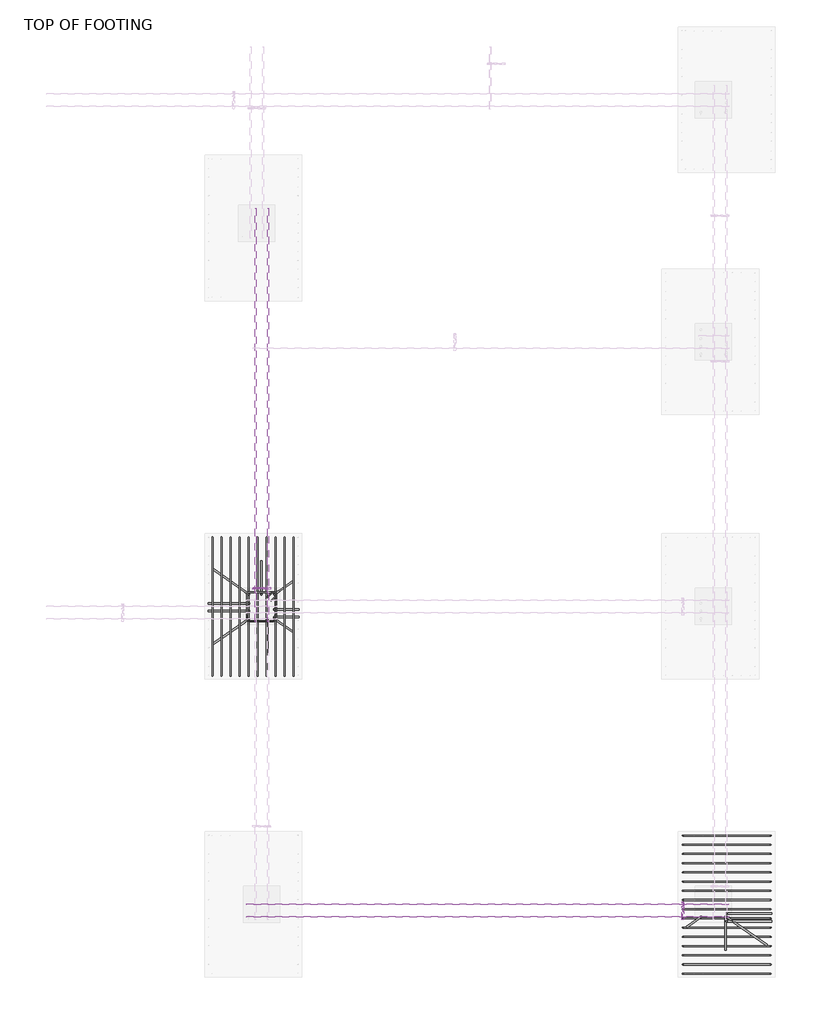
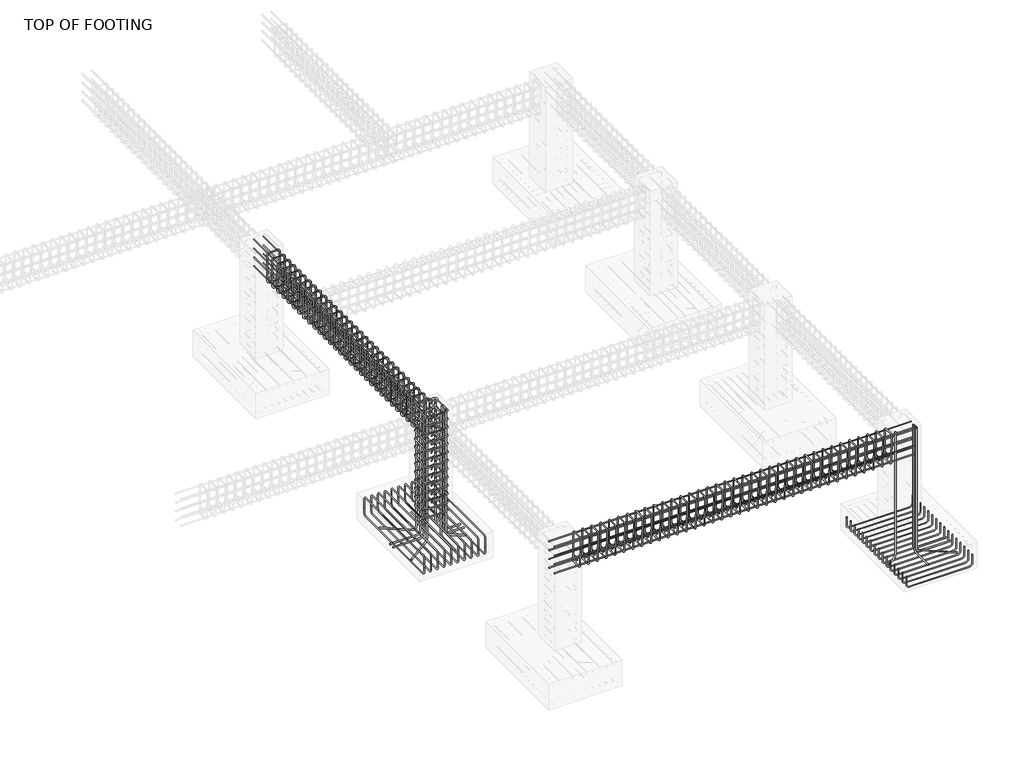
# One storey, part 4 of 11: 22 reinforcing bars.
"""IFC4 building model written with IfcOpenShell, lengths in millimetres."""

from ifc_helpers import new_model, si_unit, point, frame, origin, place, context, project, spatial, polyline, circle_curve, trimmed, segment, composite_curve, source, transform, mapped, element, save
from ifc_brep_helpers import swept_disk

model = new_model("IFC4")

# Units and contexts
model_context = context("Model", 3, world=origin())
ifc_project = project(units=[si_unit("LENGTHUNIT", "METRE", prefix="MILLI")], contexts=[model_context])

# Site, building, storey
site = spatial("IfcSite", under=ifc_project)
building = spatial("IfcBuilding", under=site)
storey = spatial("IfcBuildingStorey", under=building, Name="TOP OF FOOTING", Elevation=-1828.8)

# Reinforcing bars
placement = place(None, origin())
reinforcing_bar_shape = source(origin(), model_context, "Body", "SolidModel", [
    swept_disk(composite_curve([segment(polyline([(-1859.9394572, -2335.4013044, -2084.0984403), (-1859.9394572, -2335.4013044, -1936.7984403)]), True, "CONTINUOUS"), segment(trimmed(circle_curve(frame((-1859.9394572, -2381.7513044, -1936.7984403), z_axis=(1.0, 0.0, 0.0), x_axis=(0.0, 46.350000000000364, 0.0)), 46.35), [point((-1859.9394572, -2335.4013044, -1936.7984403))], [point((-1859.9394572, -2381.7513044, -1890.4484403))], True, "CARTESIAN"), True, "CONTINUOUS"), segment(polyline([(-1859.9394572, -2381.7513044, -1890.4484403), (-1859.9394572, -3996.3513044, -1890.4484403)]), True, "CONTINUOUS"), segment(trimmed(circle_curve(frame((-1859.9394572, -3996.3513044, -1936.7984403), z_axis=(1.0, 0.0, 0.0), x_axis=(0.0, 0.0, 46.350000000000136)), 46.35), [point((-1859.9394572, -3996.3513044, -1890.4484403))], [point((-1859.9394572, -4042.7013044, -1936.7984403))], True, "CARTESIAN"), True, "CONTINUOUS"), segment(polyline([(-1859.9394572, -4042.7013044, -1936.7984403), (-1859.9394572, -4042.7013044, -2084.0984403)]), True, "CONTINUOUS")], self_intersect=False), 6.35),
])
element("IfcReinforcingBar", 1, at=placement, inside=storey, context=model_context, shape_type="MappedRepresentation", body=[
    mapped(reinforcing_bar_shape, transform((0.0, 0.0, 0.0), x_axis=(1.0, 0.0, 0.0), y_axis=(0.0, 1.0, 0.0), z_axis=(0.0, 0.0, 1.0))),
    mapped(reinforcing_bar_shape, transform((-111.55177, 0.0, 0.0), x_axis=(1.0, 0.0, 0.0), y_axis=(0.0, 1.0, 0.0), z_axis=(0.0, 0.0, 1.0))),
    mapped(reinforcing_bar_shape, transform((-223.10354, 0.0, 0.0), x_axis=(1.0, 0.0, 0.0), y_axis=(0.0, 1.0, 0.0), z_axis=(0.0, 0.0, 1.0))),
    mapped(reinforcing_bar_shape, transform((-334.6553099, 0.0, 0.0), x_axis=(1.0, 0.0, 0.0), y_axis=(0.0, 1.0, 0.0), z_axis=(0.0, 0.0, 1.0))),
    mapped(reinforcing_bar_shape, transform((-446.2070799, 0.0, 0.0), x_axis=(1.0, 0.0, 0.0), y_axis=(0.0, 1.0, 0.0), z_axis=(0.0, 0.0, 1.0))),
    mapped(reinforcing_bar_shape, transform((-557.7588499, 0.0, 0.0), x_axis=(1.0, 0.0, 0.0), y_axis=(0.0, 1.0, 0.0), z_axis=(0.0, 0.0, 1.0))),
    mapped(reinforcing_bar_shape, transform((-669.3106199, 0.0, 0.0), x_axis=(1.0, 0.0, 0.0), y_axis=(0.0, 1.0, 0.0), z_axis=(0.0, 0.0, 1.0))),
    mapped(reinforcing_bar_shape, transform((-780.8623899, 0.0, 0.0), x_axis=(1.0, 0.0, 0.0), y_axis=(0.0, 1.0, 0.0), z_axis=(0.0, 0.0, 1.0))),
    mapped(reinforcing_bar_shape, transform((-892.4141599, 0.0, 0.0), x_axis=(1.0, 0.0, 0.0), y_axis=(0.0, 1.0, 0.0), z_axis=(0.0, 0.0, 1.0))),
    mapped(reinforcing_bar_shape, transform((-1003.9659298, 0.0, 0.0), x_axis=(1.0, 0.0, 0.0), y_axis=(0.0, 1.0, 0.0), z_axis=(0.0, 0.0, 1.0))),
])
reinforcing_bar_2_shape = source(origin(), model_context, "Body", "SolidModel", [
    swept_disk(composite_curve([segment(polyline([(-2863.9053871, -2335.4013044, -2021.5298587), (-2863.9053871, -2335.4013044, -2168.8298587)]), True, "CONTINUOUS"), segment(trimmed(circle_curve(frame((-2863.9053871, -2381.7513044, -2168.8298587), z_axis=(-1.0, 0.0, 0.0), x_axis=(0.0, 46.350000000000364, 0.0)), 46.35), [point((-2863.9053871, -2335.4013044, -2168.8298587))], [point((-2863.9053871, -2381.7513044, -2215.1798587))], True, "CARTESIAN"), True, "CONTINUOUS"), segment(polyline([(-2863.9053871, -2381.7513044, -2215.1798587), (-2863.9053871, -3996.3513044, -2215.1798587)]), True, "CONTINUOUS"), segment(trimmed(circle_curve(frame((-2863.9053871, -3996.3513044, -2168.8298587), z_axis=(-1.0, 0.0, 0.0), x_axis=(0.0, 0.0, -46.34999999999991)), 46.35), [point((-2863.9053871, -3996.3513044, -2215.1798587))], [point((-2863.9053871, -4042.7013044, -2168.8298587))], True, "CARTESIAN"), True, "CONTINUOUS"), segment(polyline([(-2863.9053871, -4042.7013044, -2168.8298587), (-2863.9053871, -4042.7013044, -2021.5298587)]), True, "CONTINUOUS")], self_intersect=False), 6.35),
])
element("IfcReinforcingBar", 2, at=placement, inside=storey, context=model_context, shape_type="MappedRepresentation", body=[
    mapped(reinforcing_bar_2_shape, transform((0.0, 0.0, 0.0), x_axis=(1.0, 0.0, 0.0), y_axis=(0.0, 1.0, 0.0), z_axis=(0.0, 0.0, 1.0))),
    mapped(reinforcing_bar_2_shape, transform((111.55177, 0.0, 0.0), x_axis=(1.0, 0.0, 0.0), y_axis=(0.0, 1.0, 0.0), z_axis=(0.0, 0.0, 1.0))),
    mapped(reinforcing_bar_2_shape, transform((223.10354, 0.0, 0.0), x_axis=(1.0, 0.0, 0.0), y_axis=(0.0, 1.0, 0.0), z_axis=(0.0, 0.0, 1.0))),
    mapped(reinforcing_bar_2_shape, transform((334.6553099, 0.0, 0.0), x_axis=(1.0, 0.0, 0.0), y_axis=(0.0, 1.0, 0.0), z_axis=(0.0, 0.0, 1.0))),
    mapped(reinforcing_bar_2_shape, transform((446.2070799, 0.0, 0.0), x_axis=(1.0, 0.0, 0.0), y_axis=(0.0, 1.0, 0.0), z_axis=(0.0, 0.0, 1.0))),
    mapped(reinforcing_bar_2_shape, transform((557.7588499, 0.0, 0.0), x_axis=(1.0, 0.0, 0.0), y_axis=(0.0, 1.0, 0.0), z_axis=(0.0, 0.0, 1.0))),
    mapped(reinforcing_bar_2_shape, transform((669.3106199, 0.0, 0.0), x_axis=(1.0, 0.0, 0.0), y_axis=(0.0, 1.0, 0.0), z_axis=(0.0, 0.0, 1.0))),
    mapped(reinforcing_bar_2_shape, transform((780.8623899, 0.0, 0.0), x_axis=(1.0, 0.0, 0.0), y_axis=(0.0, 1.0, 0.0), z_axis=(0.0, 0.0, 1.0))),
    mapped(reinforcing_bar_2_shape, transform((892.4141599, 0.0, 0.0), x_axis=(1.0, 0.0, 0.0), y_axis=(0.0, 1.0, 0.0), z_axis=(0.0, 0.0, 1.0))),
    mapped(reinforcing_bar_2_shape, transform((1003.9659298, 0.0, 0.0), x_axis=(1.0, 0.0, 0.0), y_axis=(0.0, 1.0, 0.0), z_axis=(0.0, 0.0, 1.0))),
])
reinforcing_bar_3_shape = source(origin(), model_context, "Body", "SolidModel", [
    swept_disk(composite_curve([segment(polyline([(4036.7789753, -6018.1250095, -2046.7466921), (4036.7789753, -6018.1250095, -2194.0466921)]), True, "CONTINUOUS"), segment(trimmed(circle_curve(frame((3990.4289753, -6018.1250095, -2194.0466921), z_axis=(0.0, 1.0, 0.0), x_axis=(46.350000000000364, 0.0, 0.0)), 46.35), [point((4036.7789753, -6018.1250095, -2194.0466921))], [point((3990.4289753, -6018.1250095, -2240.3966921))], True, "CARTESIAN"), True, "CONTINUOUS"), segment(polyline([(3990.4289753, -6018.1250095, -2240.3966921), (2999.2007226, -6018.1250095, -2240.3966921)]), True, "CONTINUOUS"), segment(trimmed(circle_curve(frame((2999.2007226, -6018.1250095, -2194.0466921), z_axis=(0.0, 1.0, 0.0), x_axis=(0.0, 0.0, -46.34999999999991)), 46.35), [point((2999.2007226, -6018.1250095, -2240.3966921))], [point((2952.8507226, -6018.1250095, -2194.0466921))], True, "CARTESIAN"), True, "CONTINUOUS"), segment(polyline([(2952.8507226, -6018.1250095, -2194.0466921), (2952.8507226, -6018.1250095, -2046.7466921)]), True, "CONTINUOUS")], self_intersect=False), 6.35),
])
element("IfcReinforcingBar", 3, at=placement, inside=storey, context=model_context, shape_type="MappedRepresentation", body=[
    mapped(reinforcing_bar_3_shape, transform((0.0, 0.0, 0.0), x_axis=(1.0, 0.0, 0.0), y_axis=(0.0, 1.0, 0.0), z_axis=(0.0, 0.0, 1.0))),
    mapped(reinforcing_bar_3_shape, transform((0.0, -113.82, 0.0), x_axis=(1.0, 0.0, 0.0), y_axis=(0.0, 1.0, 0.0), z_axis=(0.0, 0.0, 1.0))),
    mapped(reinforcing_bar_3_shape, transform((0.0, -227.64, 0.0), x_axis=(1.0, 0.0, 0.0), y_axis=(0.0, 1.0, 0.0), z_axis=(0.0, 0.0, 1.0))),
    mapped(reinforcing_bar_3_shape, transform((0.0, -341.46, 0.0), x_axis=(1.0, 0.0, 0.0), y_axis=(0.0, 1.0, 0.0), z_axis=(0.0, 0.0, 1.0))),
    mapped(reinforcing_bar_3_shape, transform((0.0, -455.28, 0.0), x_axis=(1.0, 0.0, 0.0), y_axis=(0.0, 1.0, 0.0), z_axis=(0.0, 0.0, 1.0))),
    mapped(reinforcing_bar_3_shape, transform((0.0, -569.1, 0.0), x_axis=(1.0, 0.0, 0.0), y_axis=(0.0, 1.0, 0.0), z_axis=(0.0, 0.0, 1.0))),
    mapped(reinforcing_bar_3_shape, transform((0.0, -682.92, 0.0), x_axis=(1.0, 0.0, 0.0), y_axis=(0.0, 1.0, 0.0), z_axis=(0.0, 0.0, 1.0))),
    mapped(reinforcing_bar_3_shape, transform((0.0, -796.74, 0.0), x_axis=(1.0, 0.0, 0.0), y_axis=(0.0, 1.0, 0.0), z_axis=(0.0, 0.0, 1.0))),
    mapped(reinforcing_bar_3_shape, transform((0.0, -910.56, 0.0), x_axis=(1.0, 0.0, 0.0), y_axis=(0.0, 1.0, 0.0), z_axis=(0.0, 0.0, 1.0))),
    mapped(reinforcing_bar_3_shape, transform((0.0, -1024.38, 0.0), x_axis=(1.0, 0.0, 0.0), y_axis=(0.0, 1.0, 0.0), z_axis=(0.0, 0.0, 1.0))),
    mapped(reinforcing_bar_3_shape, transform((0.0, -1138.2, 0.0), x_axis=(1.0, 0.0, 0.0), y_axis=(0.0, 1.0, 0.0), z_axis=(0.0, 0.0, 1.0))),
    mapped(reinforcing_bar_3_shape, transform((0.0, -1252.02, 0.0), x_axis=(1.0, 0.0, 0.0), y_axis=(0.0, 1.0, 0.0), z_axis=(0.0, 0.0, 1.0))),
    mapped(reinforcing_bar_3_shape, transform((0.0, -1365.84, 0.0), x_axis=(1.0, 0.0, 0.0), y_axis=(0.0, 1.0, 0.0), z_axis=(0.0, 0.0, 1.0))),
    mapped(reinforcing_bar_3_shape, transform((0.0, -1479.66, 0.0), x_axis=(1.0, 0.0, 0.0), y_axis=(0.0, 1.0, 0.0), z_axis=(0.0, 0.0, 1.0))),
    mapped(reinforcing_bar_3_shape, transform((0.0, -1593.48, 0.0), x_axis=(1.0, 0.0, 0.0), y_axis=(0.0, 1.0, 0.0), z_axis=(0.0, 0.0, 1.0))),
    mapped(reinforcing_bar_3_shape, transform((0.0, -1707.3, 0.0), x_axis=(1.0, 0.0, 0.0), y_axis=(0.0, 1.0, 0.0), z_axis=(0.0, 0.0, 1.0))),
])
reinforcing_bar_4_shape = source(origin(), model_context, "Body", "SolidModel", [
    swept_disk(composite_curve([segment(polyline([(3491.9271951, -6983.1823983, -40.0), (3491.9271951, -6983.1823983, -2136.75)]), True, "CONTINUOUS"), segment(trimmed(circle_curve(frame((3558.9771951, -6983.1823983, -2136.75), z_axis=(0.0, -1.0, 0.0), x_axis=(-67.04999999999973, 0.0, 0.0)), 67.05), [point((3491.9271951, -6983.1823983, -2136.75))], [point((3558.9771951, -6983.1823983, -2203.8))], True, "CARTESIAN"), True, "CONTINUOUS"), segment(polyline([(3558.9771951, -6983.1823983, -2203.8), (4054.6271951, -6983.1823983, -2203.8)]), True, "CONTINUOUS")], self_intersect=False), 9.55),
])
element("IfcReinforcingBar", 4, at=placement, inside=storey, context=model_context, shape_type="MappedRepresentation", body=[
    mapped(reinforcing_bar_4_shape, transform((0.0, 0.0, 0.0), x_axis=(1.0, 0.0, 0.0), y_axis=(0.0, 1.0, 0.0), z_axis=(0.0, 0.0, 1.0))),
    mapped(reinforcing_bar_4_shape, transform((0.0, -94.3634327, 0.0), x_axis=(1.0, 0.0, 0.0), y_axis=(0.0, 1.0, 0.0), z_axis=(0.0, 0.0, 1.0))),
])
element("IfcReinforcingBar", 5, at=placement, inside=storey, context=model_context, shape_type="SolidModel", body=[
    swept_disk(composite_curve([segment(polyline([(3491.9271951, -7022.7250095, -40.0), (3491.9271951, -7022.7250095, -2136.75)]), True, "CONTINUOUS"), segment(trimmed(circle_curve(frame((3546.8513397, -7061.1833096, -2136.75), z_axis=(-0.5735764363510477, -0.8191520442889907, 0.0), x_axis=(-54.92414460000009, 38.45830010000009, 0.0)), 67.05), [point((3491.9271951, -7022.7250095, -2136.75))], [point((3546.8513397, -7061.1833096, -2203.8))], True, "CARTESIAN"), True, "CONTINUOUS"), segment(polyline([(3546.8513397, -7061.1833096, -2203.8), (3989.9912438, -7371.4732109, -2203.8)]), True, "CONTINUOUS")], self_intersect=False), 9.55),
])
element("IfcReinforcingBar", 6, at=placement, inside=storey, context=model_context, shape_type="SolidModel", body=[
    swept_disk(composite_curve([segment(polyline([(3177.3271951, -7022.7250095, -40.0), (3177.3271951, -7022.7250095, -2136.75)]), True, "CONTINUOUS"), segment(trimmed(circle_curve(frame((3122.4030505, -7061.1833096, -2136.75), z_axis=(-0.5735764363510477, 0.8191520442889907, 0.0), x_axis=(54.92414460000009, 38.45830010000009, 0.0)), 67.05), [point((3177.3271951, -7022.7250095, -2136.75))], [point((3122.4030505, -7061.1833096, -2203.8))], True, "CARTESIAN"), True, "CONTINUOUS"), segment(polyline([(3122.4030505, -7061.1833096, -2203.8), (2999.2631464, -7147.4067987, -2203.8)]), True, "CONTINUOUS")], self_intersect=False), 9.55),
])
element("IfcReinforcingBar", 7, at=placement, inside=storey, context=model_context, shape_type="SolidModel", body=[
    swept_disk(composite_curve([segment(polyline([(3481.9271951, -7022.7250095, -40.0), (3481.9271951, -7022.7250095, -2136.75)]), True, "CONTINUOUS"), segment(trimmed(circle_curve(frame((3481.9271951, -7089.7750095, -2136.75), z_axis=(-1.0, 0.0, 0.0), x_axis=(0.0, 67.05000000000018, 0.0)), 67.05), [point((3481.9271951, -7022.7250095, -2136.75))], [point((3481.9271951, -7089.7750095, -2203.8))], True, "CARTESIAN"), True, "CONTINUOUS"), segment(polyline([(3481.9271951, -7089.7750095, -2203.8), (3481.9271951, -7435.4250095, -2203.8)]), True, "CONTINUOUS")], self_intersect=False), 9.55),
])
reinforcing_bar_5_shape = source(origin(), model_context, "Body", "SolidModel", [
    swept_disk(composite_curve([segment(polyline([(-2185.9841654, -3075.3270697, -46.35), (-2130.2406025, -3019.5835068, -46.35)]), True, "CONTINUOUS"), segment(trimmed(circle_curve(frame((-2108.0728049, -3041.7513044, -46.35), z_axis=(0.0, 0.0, -1.0), x_axis=(-22.167797600000085, 22.167797600000085, 0.0)), 31.35), [point((-2130.2406025, -3019.5835068, -46.35))], [point((-2076.7228049, -3041.7513044, -46.35))], True, "CARTESIAN"), True, "CONTINUOUS"), segment(polyline([(-2076.7228049, -3041.7513044, -46.35), (-2076.7228049, -3336.3513044, -46.35)]), True, "CONTINUOUS"), segment(trimmed(circle_curve(frame((-2108.0728049, -3336.3513044, -46.35), z_axis=(0.0, 0.0, -1.0), x_axis=(31.34999999999991, 0.0, 0.0)), 31.35), [point((-2076.7228049, -3336.3513044, -46.35))], [point((-2108.0728049, -3367.7013044, -46.35))], True, "CARTESIAN"), True, "CONTINUOUS"), segment(polyline([(-2108.0728049, -3367.7013044, -46.35), (-2402.6728049, -3367.7013044, -46.35)]), True, "CONTINUOUS"), segment(trimmed(circle_curve(frame((-2402.6728049, -3336.3710895, -45.2363875), z_axis=(0.0, 0.03552192833448185, -0.9993688971583016), x_axis=(0.0, -31.3302149000001, -1.1136125000000021)), 31.35), [point((-2402.6728049, -3367.7013044, -46.35))], [point((-2434.0228049, -3336.3710895, -45.2363875))], True, "CARTESIAN"), True, "CONTINUOUS"), segment(polyline([(-2434.0228049, -3336.3710895, -45.2363875), (-2434.0228049, -3041.7315193, -34.7636125)]), True, "CONTINUOUS"), segment(trimmed(circle_curve(frame((-2402.6728049, -3041.7315193, -34.7636125), z_axis=(0.0, 0.03552192833448185, -0.9993688971583016), x_axis=(-31.350000000000364, 0.0, 0.0)), 31.35), [point((-2434.0228049, -3041.7315193, -34.7636125))], [point((-2402.6728049, -3010.4013044, -33.65))], True, "CARTESIAN"), True, "CONTINUOUS"), segment(polyline([(-2402.6728049, -3010.4013044, -33.65), (-2108.0728049, -3010.4013044, -33.65)]), True, "CONTINUOUS"), segment(trimmed(circle_curve(frame((-2108.0728049, -3041.7513044, -33.65), z_axis=(0.0, 0.0, -1.0), x_axis=(0.0, 31.350000000000364, 0.0)), 31.35), [point((-2108.0728049, -3010.4013044, -33.65))], [point((-2085.9050073, -3063.919102, -33.65))], True, "CARTESIAN"), True, "CONTINUOUS"), segment(polyline([(-2085.9050073, -3063.919102, -33.65), (-2141.6485703, -3119.6626649, -33.65)]), True, "CONTINUOUS")], self_intersect=False), 6.35),
])
element("IfcReinforcingBar", 8, at=placement, inside=storey, context=model_context, shape_type="MappedRepresentation", body=[
    mapped(reinforcing_bar_5_shape, transform((0.0, 0.0, 0.0), x_axis=(1.0, 0.0, 0.0), y_axis=(0.0, 1.0, 0.0), z_axis=(0.0, 0.0, 1.0))),
    mapped(reinforcing_bar_5_shape, transform((0.0, 0.0, -144.675), x_axis=(1.0, 0.0, 0.0), y_axis=(0.0, 1.0, 0.0), z_axis=(0.0, 0.0, 1.0))),
    mapped(reinforcing_bar_5_shape, transform((0.0, 0.0, -289.35), x_axis=(1.0, 0.0, 0.0), y_axis=(0.0, 1.0, 0.0), z_axis=(0.0, 0.0, 1.0))),
    mapped(reinforcing_bar_5_shape, transform((0.0, 0.0, -434.025), x_axis=(1.0, 0.0, 0.0), y_axis=(0.0, 1.0, 0.0), z_axis=(0.0, 0.0, 1.0))),
    mapped(reinforcing_bar_5_shape, transform((0.0, 0.0, -578.7), x_axis=(1.0, 0.0, 0.0), y_axis=(0.0, 1.0, 0.0), z_axis=(0.0, 0.0, 1.0))),
    mapped(reinforcing_bar_5_shape, transform((0.0, 0.0, -723.375), x_axis=(1.0, 0.0, 0.0), y_axis=(0.0, 1.0, 0.0), z_axis=(0.0, 0.0, 1.0))),
    mapped(reinforcing_bar_5_shape, transform((0.0, 0.0, -868.05), x_axis=(1.0, 0.0, 0.0), y_axis=(0.0, 1.0, 0.0), z_axis=(0.0, 0.0, 1.0))),
    mapped(reinforcing_bar_5_shape, transform((0.0, 0.0, -1012.725), x_axis=(1.0, 0.0, 0.0), y_axis=(0.0, 1.0, 0.0), z_axis=(0.0, 0.0, 1.0))),
    mapped(reinforcing_bar_5_shape, transform((0.0, 0.0, -1157.4), x_axis=(1.0, 0.0, 0.0), y_axis=(0.0, 1.0, 0.0), z_axis=(0.0, 0.0, 1.0))),
    mapped(reinforcing_bar_5_shape, transform((0.0, 0.0, -1302.075), x_axis=(1.0, 0.0, 0.0), y_axis=(0.0, 1.0, 0.0), z_axis=(0.0, 0.0, 1.0))),
    mapped(reinforcing_bar_5_shape, transform((0.0, 0.0, -1446.75), x_axis=(1.0, 0.0, 0.0), y_axis=(0.0, 1.0, 0.0), z_axis=(0.0, 0.0, 1.0))),
    mapped(reinforcing_bar_5_shape, transform((0.0, 0.0, -1591.425), x_axis=(1.0, 0.0, 0.0), y_axis=(0.0, 1.0, 0.0), z_axis=(0.0, 0.0, 1.0))),
    mapped(reinforcing_bar_5_shape, transform((0.0, 0.0, -1736.1), x_axis=(1.0, 0.0, 0.0), y_axis=(0.0, 1.0, 0.0), z_axis=(0.0, 0.0, 1.0))),
])
reinforcing_bar_6_shape = source(origin(), model_context, "Body", "SolidModel", [
    swept_disk(composite_curve([segment(polyline([(-2098.0728049, -3225.4586931, -40.0), (-2098.0728049, -3225.4586931, -2136.75)]), True, "CONTINUOUS"), segment(trimmed(circle_curve(frame((-2031.0228049, -3225.4586931, -2136.75), z_axis=(0.0, -1.0, 0.0), x_axis=(-67.04999999999995, 0.0, 0.0)), 67.05), [point((-2098.0728049, -3225.4586931, -2136.75))], [point((-2031.0228049, -3225.4586931, -2203.8))], True, "CARTESIAN"), True, "CONTINUOUS"), segment(polyline([(-2031.0228049, -3225.4586931, -2203.8), (-1795.3728049, -3225.4586931, -2203.8)]), True, "CONTINUOUS")], self_intersect=False), 9.55),
])
element("IfcReinforcingBar", 9, at=placement, inside=storey, context=model_context, shape_type="MappedRepresentation", body=[
    mapped(reinforcing_bar_6_shape, transform((0.0, 0.0, 0.0), x_axis=(1.0, 0.0, 0.0), y_axis=(0.0, 1.0, 0.0), z_axis=(0.0, 0.0, 1.0))),
    mapped(reinforcing_bar_6_shape, transform((0.0, -94.3634327, 0.0), x_axis=(1.0, 0.0, 0.0), y_axis=(0.0, 1.0, 0.0), z_axis=(0.0, 0.0, 1.0))),
])
element("IfcReinforcingBar", 10, at=placement, inside=storey, context=model_context, shape_type="SolidModel", body=[
    swept_disk(composite_curve([segment(polyline([(-2098.0728049, -3340.0013044, -40.0), (-2098.0728049, -3340.0013044, -2136.75)]), True, "CONTINUOUS"), segment(trimmed(circle_curve(frame((-2043.1486603, -3378.4596044, -2136.75), z_axis=(-0.5735764363510477, -0.8191520442889907, 0.0), x_axis=(-54.92414459999986, 38.45829999999978, 0.0)), 67.05), [point((-2098.0728049, -3340.0013044, -2136.75))], [point((-2043.1486603, -3378.4596044, -2203.8))], True, "CARTESIAN"), True, "CONTINUOUS"), segment(polyline([(-2043.1486603, -3378.4596044, -2203.8), (-1860.0087562, -3506.6955459, -2203.8)]), True, "CONTINUOUS")], self_intersect=False), 9.55),
])
element("IfcReinforcingBar", 11, at=placement, inside=storey, context=model_context, shape_type="SolidModel", body=[
    swept_disk(composite_curve([segment(polyline([(-2098.0728049, -3038.1013044, -40.0), (-2098.0728049, -3038.1013044, -2136.75)]), True, "CONTINUOUS"), segment(trimmed(circle_curve(frame((-2043.1486603, -2999.6430043, -2136.75), z_axis=(0.5735764363510477, -0.8191520442889907, 0.0), x_axis=(-54.92414459999986, -38.45830010000009, 0.0)), 67.05), [point((-2098.0728049, -3038.1013044, -2136.75))], [point((-2043.1486603, -2999.6430043, -2203.8))], True, "CARTESIAN"), True, "CONTINUOUS"), segment(polyline([(-2043.1486603, -2999.6430043, -2203.8), (-1860.0087562, -2871.4070629, -2203.8)]), True, "CONTINUOUS")], self_intersect=False), 9.55),
])
element("IfcReinforcingBar", 12, at=placement, inside=storey, context=model_context, shape_type="SolidModel", body=[
    swept_disk(composite_curve([segment(polyline([(-2412.6728049, -3340.0013044, -40.0), (-2412.6728049, -3340.0013044, -2136.75)]), True, "CONTINUOUS"), segment(trimmed(circle_curve(frame((-2467.5969495, -3378.4596044, -2136.75), z_axis=(-0.5735764363510477, 0.8191520442889908, 0.0), x_axis=(54.92414460000009, 38.45829999999978, 0.0)), 67.05), [point((-2412.6728049, -3340.0013044, -2136.75))], [point((-2467.5969495, -3378.4596044, -2203.8))], True, "CARTESIAN"), True, "CONTINUOUS"), segment(polyline([(-2467.5969495, -3378.4596044, -2203.8), (-2850.7368536, -3646.7370535, -2203.8)]), True, "CONTINUOUS")], self_intersect=False), 9.55),
])
element("IfcReinforcingBar", 13, at=placement, inside=storey, context=model_context, shape_type="SolidModel", body=[
    swept_disk(composite_curve([segment(polyline([(-2412.6728049, -3038.1013044, -40.0), (-2412.6728049, -3038.1013044, -2136.75)]), True, "CONTINUOUS"), segment(trimmed(circle_curve(frame((-2467.5969495, -2999.6430043, -2136.75), z_axis=(0.5735764363510478, 0.8191520442889907, 0.0), x_axis=(54.92414460000009, -38.45830010000009, 0.0)), 67.05), [point((-2412.6728049, -3038.1013044, -2136.75))], [point((-2467.5969495, -2999.6430043, -2203.8))], True, "CARTESIAN"), True, "CONTINUOUS"), segment(polyline([(-2467.5969495, -2999.6430043, -2203.8), (-2850.7368536, -2731.3655553, -2203.8)]), True, "CONTINUOUS")], self_intersect=False), 9.55),
])
reinforcing_bar_7_shape = source(origin(), model_context, "Body", "SolidModel", [
    swept_disk(composite_curve([segment(polyline([(-2412.6728049, -3150.4586931, -40.0), (-2412.6728049, -3150.4586931, -2136.75)]), True, "CONTINUOUS"), segment(trimmed(circle_curve(frame((-2479.7228049, -3150.4586931, -2136.75), z_axis=(0.0, 1.0, 0.0), x_axis=(67.05000000000018, 0.0, 0.0)), 67.05), [point((-2412.6728049, -3150.4586931, -2136.75))], [point((-2479.7228049, -3150.4586931, -2203.8))], True, "CARTESIAN"), True, "CONTINUOUS"), segment(polyline([(-2479.7228049, -3150.4586931, -2203.8), (-2915.3728049, -3150.4586931, -2203.8)]), True, "CONTINUOUS")], self_intersect=False), 9.55),
])
element("IfcReinforcingBar", 14, at=placement, inside=storey, context=model_context, shape_type="MappedRepresentation", body=[
    mapped(reinforcing_bar_7_shape, transform((0.0, 0.0, 0.0), x_axis=(1.0, 0.0, 0.0), y_axis=(0.0, 1.0, 0.0), z_axis=(0.0, 0.0, 1.0))),
    mapped(reinforcing_bar_7_shape, transform((0.0, -94.3634327, 0.0), x_axis=(1.0, 0.0, 0.0), y_axis=(0.0, 1.0, 0.0), z_axis=(0.0, 0.0, 1.0))),
])
element("IfcReinforcingBar", 15, at=placement, inside=storey, context=model_context, shape_type="SolidModel", body=[
    swept_disk(composite_curve([segment(polyline([(-2258.0728049, -3038.1013044, -40.0), (-2258.0728049, -3038.1013044, -2136.75)]), True, "CONTINUOUS"), segment(trimmed(circle_curve(frame((-2258.0728049, -2971.0513044, -2136.75), z_axis=(1.0, 0.0, 0.0), x_axis=(0.0, -67.05000000000018, 0.0)), 67.05), [point((-2258.0728049, -3038.1013044, -2136.75))], [point((-2258.0728049, -2971.0513044, -2203.8))], True, "CARTESIAN"), True, "CONTINUOUS"), segment(polyline([(-2258.0728049, -2971.0513044, -2203.8), (-2258.0728049, -2625.4013044, -2203.8)]), True, "CONTINUOUS")], self_intersect=False), 9.55),
])
element("IfcReinforcingBar", 16, at=placement, inside=storey, context=model_context, shape_type="SolidModel", body=[
    swept_disk(composite_curve([segment(polyline([(-2183.0728049, -3340.0013044, -40.0), (-2183.0728049, -3340.0013044, -2136.75)]), True, "CONTINUOUS"), segment(trimmed(circle_curve(frame((-2183.0728049, -3407.0513044, -2136.75), z_axis=(-1.0, 0.0, 0.0), x_axis=(0.0, 67.04999999999973, 0.0)), 67.05), [point((-2183.0728049, -3340.0013044, -2136.75))], [point((-2183.0728049, -3407.0513044, -2203.8))], True, "CARTESIAN"), True, "CONTINUOUS"), segment(polyline([(-2183.0728049, -3407.0513044, -2203.8), (-2183.0728049, -3752.7013044, -2203.8)]), True, "CONTINUOUS")], self_intersect=False), 9.55),
])
reinforcing_bar_8_shape = source(origin(), model_context, "Body", "SolidModel", [
    swept_disk(composite_curve([segment(polyline([(-2249.7614444, -2957.7013044, -488.7242346), (-2305.5050073, -2957.7013044, -544.4677976)]), True, "CONTINUOUS"), segment(trimmed(circle_curve(frame((-2327.6728049, -2957.7013044, -522.3), z_axis=(0.0, 1.0, 0.0), x_axis=(22.16779759999963, 0.0, -22.167797600000085)), 31.35), [point((-2305.5050073, -2957.7013044, -544.4677976))], [point((-2359.0228049, -2957.7013044, -522.3))], True, "CARTESIAN"), True, "CONTINUOUS"), segment(polyline([(-2359.0228049, -2957.7013044, -522.3), (-2359.0228049, -2957.7013044, -77.7)]), True, "CONTINUOUS"), segment(trimmed(circle_curve(frame((-2327.6728049, -2957.7013044, -77.7), z_axis=(0.0, 1.0, 0.0), x_axis=(-31.350000000000364, 0.0, 0.0)), 31.35), [point((-2359.0228049, -2957.7013044, -77.7))], [point((-2327.6728049, -2957.7013044, -46.35))], True, "CARTESIAN"), True, "CONTINUOUS"), segment(polyline([(-2327.6728049, -2957.7013044, -46.35), (-2183.0728049, -2957.7013044, -46.35)]), True, "CONTINUOUS"), segment(trimmed(circle_curve(frame((-2183.0728049, -2958.48589, -77.6901807), z_axis=(0.0, 0.9996867842138424, -0.025026655153786322), x_axis=(0.0, 0.7845855999999003, 31.340180699999998)), 31.35), [point((-2183.0728049, -2957.7013044, -46.35))], [point((-2151.7228049, -2958.48589, -77.6901807))], True, "CARTESIAN"), True, "CONTINUOUS"), segment(polyline([(-2151.7228049, -2958.48589, -77.6901807), (-2151.7228049, -2969.6167188, -522.3098193)]), True, "CONTINUOUS"), segment(trimmed(circle_curve(frame((-2183.0728049, -2969.6167188, -522.3098193), z_axis=(0.0, 0.9996867842138424, -0.025026655153786322), x_axis=(31.34999999999991, 0.0, 0.0)), 31.35), [point((-2151.7228049, -2969.6167188, -522.3098193))], [point((-2183.0728049, -2970.4013044, -553.65))], True, "CARTESIAN"), True, "CONTINUOUS"), segment(polyline([(-2183.0728049, -2970.4013044, -553.65), (-2327.6728049, -2970.4013044, -553.65)]), True, "CONTINUOUS"), segment(trimmed(circle_curve(frame((-2327.6728049, -2970.4013044, -522.3), z_axis=(0.0, 1.0, 0.0), x_axis=(0.0, 0.0, -31.350000000000023)), 31.35), [point((-2327.6728049, -2970.4013044, -553.65))], [point((-2349.8406025, -2970.4013044, -500.1322024))], True, "CARTESIAN"), True, "CONTINUOUS"), segment(polyline([(-2349.8406025, -2970.4013044, -500.1322024), (-2294.0970395, -2970.4013044, -444.3886395)]), True, "CONTINUOUS")], self_intersect=False), 6.35),
])
element("IfcReinforcingBar", 17, at=placement, inside=storey, context=model_context, shape_type="MappedRepresentation", body=[
    mapped(reinforcing_bar_8_shape, transform((0.0, 0.0, 0.0), x_axis=(1.0, 0.0, 0.0), y_axis=(0.0, 1.0, 0.0), z_axis=(0.0, 0.0, 1.0))),
    mapped(reinforcing_bar_8_shape, transform((0.0, 147.3101511, 0.0), x_axis=(1.0, 0.0, 0.0), y_axis=(0.0, 1.0, 0.0), z_axis=(0.0, 0.0, 1.0))),
    mapped(reinforcing_bar_8_shape, transform((0.0, 294.6203023, 0.0), x_axis=(1.0, 0.0, 0.0), y_axis=(0.0, 1.0, 0.0), z_axis=(0.0, 0.0, 1.0))),
    mapped(reinforcing_bar_8_shape, transform((0.0, 441.9304534, 0.0), x_axis=(1.0, 0.0, 0.0), y_axis=(0.0, 1.0, 0.0), z_axis=(0.0, 0.0, 1.0))),
    mapped(reinforcing_bar_8_shape, transform((0.0, 589.2406046, 0.0), x_axis=(1.0, 0.0, 0.0), y_axis=(0.0, 1.0, 0.0), z_axis=(0.0, 0.0, 1.0))),
    mapped(reinforcing_bar_8_shape, transform((0.0, 736.5507557, 0.0), x_axis=(1.0, 0.0, 0.0), y_axis=(0.0, 1.0, 0.0), z_axis=(0.0, 0.0, 1.0))),
    mapped(reinforcing_bar_8_shape, transform((0.0, 883.8609068, 0.0), x_axis=(1.0, 0.0, 0.0), y_axis=(0.0, 1.0, 0.0), z_axis=(0.0, 0.0, 1.0))),
    mapped(reinforcing_bar_8_shape, transform((0.0, 1031.171058, 0.0), x_axis=(1.0, 0.0, 0.0), y_axis=(0.0, 1.0, 0.0), z_axis=(0.0, 0.0, 1.0))),
    mapped(reinforcing_bar_8_shape, transform((0.0, 1178.4812091, 0.0), x_axis=(1.0, 0.0, 0.0), y_axis=(0.0, 1.0, 0.0), z_axis=(0.0, 0.0, 1.0))),
    mapped(reinforcing_bar_8_shape, transform((0.0, 1325.7913603, 0.0), x_axis=(1.0, 0.0, 0.0), y_axis=(0.0, 1.0, 0.0), z_axis=(0.0, 0.0, 1.0))),
    mapped(reinforcing_bar_8_shape, transform((0.0, 1473.1015114, 0.0), x_axis=(1.0, 0.0, 0.0), y_axis=(0.0, 1.0, 0.0), z_axis=(0.0, 0.0, 1.0))),
    mapped(reinforcing_bar_8_shape, transform((0.0, 1620.4116626, 0.0), x_axis=(1.0, 0.0, 0.0), y_axis=(0.0, 1.0, 0.0), z_axis=(0.0, 0.0, 1.0))),
    mapped(reinforcing_bar_8_shape, transform((0.0, 1767.7218137, 0.0), x_axis=(1.0, 0.0, 0.0), y_axis=(0.0, 1.0, 0.0), z_axis=(0.0, 0.0, 1.0))),
    mapped(reinforcing_bar_8_shape, transform((0.0, 1915.0319648, 0.0), x_axis=(1.0, 0.0, 0.0), y_axis=(0.0, 1.0, 0.0), z_axis=(0.0, 0.0, 1.0))),
    mapped(reinforcing_bar_8_shape, transform((0.0, 2062.342116, 0.0), x_axis=(1.0, 0.0, 0.0), y_axis=(0.0, 1.0, 0.0), z_axis=(0.0, 0.0, 1.0))),
    mapped(reinforcing_bar_8_shape, transform((0.0, 2209.6522671, 0.0), x_axis=(1.0, 0.0, 0.0), y_axis=(0.0, 1.0, 0.0), z_axis=(0.0, 0.0, 1.0))),
    mapped(reinforcing_bar_8_shape, transform((0.0, 2356.9624183, 0.0), x_axis=(1.0, 0.0, 0.0), y_axis=(0.0, 1.0, 0.0), z_axis=(0.0, 0.0, 1.0))),
    mapped(reinforcing_bar_8_shape, transform((0.0, 2504.2725694, 0.0), x_axis=(1.0, 0.0, 0.0), y_axis=(0.0, 1.0, 0.0), z_axis=(0.0, 0.0, 1.0))),
    mapped(reinforcing_bar_8_shape, transform((0.0, 2651.5827205, 0.0), x_axis=(1.0, 0.0, 0.0), y_axis=(0.0, 1.0, 0.0), z_axis=(0.0, 0.0, 1.0))),
    mapped(reinforcing_bar_8_shape, transform((0.0, 2798.8928717, 0.0), x_axis=(1.0, 0.0, 0.0), y_axis=(0.0, 1.0, 0.0), z_axis=(0.0, 0.0, 1.0))),
    mapped(reinforcing_bar_8_shape, transform((0.0, 2946.2030228, 0.0), x_axis=(1.0, 0.0, 0.0), y_axis=(0.0, 1.0, 0.0), z_axis=(0.0, 0.0, 1.0))),
    mapped(reinforcing_bar_8_shape, transform((0.0, 3093.513174, 0.0), x_axis=(1.0, 0.0, 0.0), y_axis=(0.0, 1.0, 0.0), z_axis=(0.0, 0.0, 1.0))),
    mapped(reinforcing_bar_8_shape, transform((0.0, 3240.8233251, 0.0), x_axis=(1.0, 0.0, 0.0), y_axis=(0.0, 1.0, 0.0), z_axis=(0.0, 0.0, 1.0))),
    mapped(reinforcing_bar_8_shape, transform((0.0, 3388.1334762, 0.0), x_axis=(1.0, 0.0, 0.0), y_axis=(0.0, 1.0, 0.0), z_axis=(0.0, 0.0, 1.0))),
    mapped(reinforcing_bar_8_shape, transform((0.0, 3535.4436274, 0.0), x_axis=(1.0, 0.0, 0.0), y_axis=(0.0, 1.0, 0.0), z_axis=(0.0, 0.0, 1.0))),
    mapped(reinforcing_bar_8_shape, transform((0.0, 3682.7537785, 0.0), x_axis=(1.0, 0.0, 0.0), y_axis=(0.0, 1.0, 0.0), z_axis=(0.0, 0.0, 1.0))),
    mapped(reinforcing_bar_8_shape, transform((0.0, 3830.0639297, 0.0), x_axis=(1.0, 0.0, 0.0), y_axis=(0.0, 1.0, 0.0), z_axis=(0.0, 0.0, 1.0))),
    mapped(reinforcing_bar_8_shape, transform((0.0, 3977.3740808, 0.0), x_axis=(1.0, 0.0, 0.0), y_axis=(0.0, 1.0, 0.0), z_axis=(0.0, 0.0, 1.0))),
    mapped(reinforcing_bar_8_shape, transform((0.0, 4124.6842319, 0.0), x_axis=(1.0, 0.0, 0.0), y_axis=(0.0, 1.0, 0.0), z_axis=(0.0, 0.0, 1.0))),
    mapped(reinforcing_bar_8_shape, transform((0.0, 4271.9943831, 0.0), x_axis=(1.0, 0.0, 0.0), y_axis=(0.0, 1.0, 0.0), z_axis=(0.0, 0.0, 1.0))),
])
reinforcing_bar_9_shape = source(origin(), model_context, "Body", "SolidModel", [
    swept_disk(composite_curve([segment(polyline([(-2332.6728049, -3374.0513044, -528.2977114), (-2332.6728049, 1730.6430781, -528.2977114)]), True, "CONTINUOUS")], self_intersect=False), 6.35),
])
element("IfcReinforcingBar", 18, at=placement, inside=storey, context=model_context, shape_type="MappedRepresentation", body=[
    mapped(reinforcing_bar_9_shape, transform((0.0, 0.0, 0.0), x_axis=(1.0, 0.0, 0.0), y_axis=(0.0, 1.0, 0.0), z_axis=(0.0, 0.0, 1.0))),
    mapped(reinforcing_bar_9_shape, transform((0.0, 0.0, 153.3723948), x_axis=(1.0, 0.0, 0.0), y_axis=(0.0, 1.0, 0.0), z_axis=(0.0, 0.0, 1.0))),
    mapped(reinforcing_bar_9_shape, transform((0.0, 0.0, 306.7447895), x_axis=(1.0, 0.0, 0.0), y_axis=(0.0, 1.0, 0.0), z_axis=(0.0, 0.0, 1.0))),
    mapped(reinforcing_bar_9_shape, transform((0.0, 0.0, 460.1171843), x_axis=(1.0, 0.0, 0.0), y_axis=(0.0, 1.0, 0.0), z_axis=(0.0, 0.0, 1.0))),
])
reinforcing_bar_10_shape = source(origin(), model_context, "Body", "SolidModel", [
    swept_disk(composite_curve([segment(polyline([(-2178.0728049, -3374.0513044, -528.2977114), (-2178.0728049, 1730.6430781, -528.2977114)]), True, "CONTINUOUS")], self_intersect=False), 6.35),
])
element("IfcReinforcingBar", 19, at=placement, inside=storey, context=model_context, shape_type="MappedRepresentation", body=[
    mapped(reinforcing_bar_10_shape, transform((0.0, 0.0, 0.0), x_axis=(1.0, 0.0, 0.0), y_axis=(0.0, 1.0, 0.0), z_axis=(0.0, 0.0, 1.0))),
    mapped(reinforcing_bar_10_shape, transform((0.0, 0.0, 153.3723948), x_axis=(1.0, 0.0, 0.0), y_axis=(0.0, 1.0, 0.0), z_axis=(0.0, 0.0, 1.0))),
    mapped(reinforcing_bar_10_shape, transform((0.0, 0.0, 306.7447895), x_axis=(1.0, 0.0, 0.0), y_axis=(0.0, 1.0, 0.0), z_axis=(0.0, 0.0, 1.0))),
    mapped(reinforcing_bar_10_shape, transform((0.0, 0.0, 460.1171843), x_axis=(1.0, 0.0, 0.0), y_axis=(0.0, 1.0, 0.0), z_axis=(0.0, 0.0, 1.0))),
])
reinforcing_bar_11_shape = source(origin(), model_context, "Body", "SolidModel", [
    swept_disk(composite_curve([segment(polyline([(-2024.0228049, -6952.3863701, -488.7242346), (-2024.0228049, -6896.6428071, -544.4677976)]), True, "CONTINUOUS"), segment(trimmed(circle_curve(frame((-2024.0228049, -6874.4750095, -522.3), z_axis=(1.0, 0.0, 0.0), x_axis=(0.0, -22.167797600000085, -22.167797600000085)), 31.35), [point((-2024.0228049, -6896.6428071, -544.4677976))], [point((-2024.0228049, -6843.1250095, -522.3))], True, "CARTESIAN"), True, "CONTINUOUS"), segment(polyline([(-2024.0228049, -6843.1250095, -522.3), (-2024.0228049, -6843.1250095, -77.7)]), True, "CONTINUOUS"), segment(trimmed(circle_curve(frame((-2024.0228049, -6874.4750095, -77.7), z_axis=(1.0, 0.0, 0.0), x_axis=(0.0, 31.350000000000364, 0.0)), 31.35), [point((-2024.0228049, -6843.1250095, -77.7))], [point((-2024.0228049, -6874.4750095, -46.35))], True, "CARTESIAN"), True, "CONTINUOUS"), segment(polyline([(-2024.0228049, -6874.4750095, -46.35), (-2024.0228049, -7019.0750095, -46.35)]), True, "CONTINUOUS"), segment(trimmed(circle_curve(frame((-2024.8073905, -7019.0750095, -77.6901807), z_axis=(0.9996867842138424, 0.0, -0.025026655153786322), x_axis=(0.7845856000001277, 0.0, 31.340180699999998)), 31.35), [point((-2024.0228049, -7019.0750095, -46.35))], [point((-2024.8073905, -7050.4250095, -77.6901807))], True, "CARTESIAN"), True, "CONTINUOUS"), segment(polyline([(-2024.8073905, -7050.4250095, -77.6901807), (-2035.9382193, -7050.4250095, -522.3098193)]), True, "CONTINUOUS"), segment(trimmed(circle_curve(frame((-2035.9382193, -7019.0750095, -522.3098193), z_axis=(0.9996867842138424, 0.0, -0.025026655153786322), x_axis=(0.0, -31.349999999999454, 0.0)), 31.35), [point((-2035.9382193, -7050.4250095, -522.3098193))], [point((-2036.7228049, -7019.0750095, -553.65))], True, "CARTESIAN"), True, "CONTINUOUS"), segment(polyline([(-2036.7228049, -7019.0750095, -553.65), (-2036.7228049, -6874.4750095, -553.65)]), True, "CONTINUOUS"), segment(trimmed(circle_curve(frame((-2036.7228049, -6874.4750095, -522.3), z_axis=(1.0, 0.0, 0.0), x_axis=(0.0, 0.0, -31.350000000000023)), 31.35), [point((-2036.7228049, -6874.4750095, -553.65))], [point((-2036.7228049, -6852.3072119, -500.1322024))], True, "CARTESIAN"), True, "CONTINUOUS"), segment(polyline([(-2036.7228049, -6852.3072119, -500.1322024), (-2036.7228049, -6908.0507749, -444.3886395)]), True, "CONTINUOUS")], self_intersect=False), 6.35),
])
element("IfcReinforcingBar", 20, at=placement, inside=storey, context=model_context, shape_type="MappedRepresentation", body=[
    mapped(reinforcing_bar_11_shape, transform((0.0, 0.0, 0.0), x_axis=(1.0, 0.0, 0.0), y_axis=(0.0, 1.0, 0.0), z_axis=(0.0, 0.0, 1.0))),
    mapped(reinforcing_bar_11_shape, transform((146.4942857, 0.0, 0.0), x_axis=(1.0, 0.0, 0.0), y_axis=(0.0, 1.0, 0.0), z_axis=(0.0, 0.0, 1.0))),
    mapped(reinforcing_bar_11_shape, transform((292.9885714, 0.0, 0.0), x_axis=(1.0, 0.0, 0.0), y_axis=(0.0, 1.0, 0.0), z_axis=(0.0, 0.0, 1.0))),
    mapped(reinforcing_bar_11_shape, transform((439.4828571, 0.0, 0.0), x_axis=(1.0, 0.0, 0.0), y_axis=(0.0, 1.0, 0.0), z_axis=(0.0, 0.0, 1.0))),
    mapped(reinforcing_bar_11_shape, transform((585.9771429, 0.0, 0.0), x_axis=(1.0, 0.0, 0.0), y_axis=(0.0, 1.0, 0.0), z_axis=(0.0, 0.0, 1.0))),
    mapped(reinforcing_bar_11_shape, transform((732.4714286, 0.0, 0.0), x_axis=(1.0, 0.0, 0.0), y_axis=(0.0, 1.0, 0.0), z_axis=(0.0, 0.0, 1.0))),
    mapped(reinforcing_bar_11_shape, transform((878.9657143, 0.0, 0.0), x_axis=(1.0, 0.0, 0.0), y_axis=(0.0, 1.0, 0.0), z_axis=(0.0, 0.0, 1.0))),
    mapped(reinforcing_bar_11_shape, transform((1025.46, 0.0, 0.0), x_axis=(1.0, 0.0, 0.0), y_axis=(0.0, 1.0, 0.0), z_axis=(0.0, 0.0, 1.0))),
    mapped(reinforcing_bar_11_shape, transform((1171.9542857, 0.0, 0.0), x_axis=(1.0, 0.0, 0.0), y_axis=(0.0, 1.0, 0.0), z_axis=(0.0, 0.0, 1.0))),
    mapped(reinforcing_bar_11_shape, transform((1318.4485714, 0.0, 0.0), x_axis=(1.0, 0.0, 0.0), y_axis=(0.0, 1.0, 0.0), z_axis=(0.0, 0.0, 1.0))),
    mapped(reinforcing_bar_11_shape, transform((1464.9428571, 0.0, 0.0), x_axis=(1.0, 0.0, 0.0), y_axis=(0.0, 1.0, 0.0), z_axis=(0.0, 0.0, 1.0))),
    mapped(reinforcing_bar_11_shape, transform((1611.4371429, 0.0, 0.0), x_axis=(1.0, 0.0, 0.0), y_axis=(0.0, 1.0, 0.0), z_axis=(0.0, 0.0, 1.0))),
    mapped(reinforcing_bar_11_shape, transform((1757.9314286, 0.0, 0.0), x_axis=(1.0, 0.0, 0.0), y_axis=(0.0, 1.0, 0.0), z_axis=(0.0, 0.0, 1.0))),
    mapped(reinforcing_bar_11_shape, transform((1904.4257143, 0.0, 0.0), x_axis=(1.0, 0.0, 0.0), y_axis=(0.0, 1.0, 0.0), z_axis=(0.0, 0.0, 1.0))),
    mapped(reinforcing_bar_11_shape, transform((2050.92, 0.0, 0.0), x_axis=(1.0, 0.0, 0.0), y_axis=(0.0, 1.0, 0.0), z_axis=(0.0, 0.0, 1.0))),
    mapped(reinforcing_bar_11_shape, transform((2197.4142857, 0.0, 0.0), x_axis=(1.0, 0.0, 0.0), y_axis=(0.0, 1.0, 0.0), z_axis=(0.0, 0.0, 1.0))),
    mapped(reinforcing_bar_11_shape, transform((2343.9085714, 0.0, 0.0), x_axis=(1.0, 0.0, 0.0), y_axis=(0.0, 1.0, 0.0), z_axis=(0.0, 0.0, 1.0))),
    mapped(reinforcing_bar_11_shape, transform((2490.4028571, 0.0, 0.0), x_axis=(1.0, 0.0, 0.0), y_axis=(0.0, 1.0, 0.0), z_axis=(0.0, 0.0, 1.0))),
    mapped(reinforcing_bar_11_shape, transform((2636.8971429, 0.0, 0.0), x_axis=(1.0, 0.0, 0.0), y_axis=(0.0, 1.0, 0.0), z_axis=(0.0, 0.0, 1.0))),
    mapped(reinforcing_bar_11_shape, transform((2783.3914286, 0.0, 0.0), x_axis=(1.0, 0.0, 0.0), y_axis=(0.0, 1.0, 0.0), z_axis=(0.0, 0.0, 1.0))),
    mapped(reinforcing_bar_11_shape, transform((2929.8857143, 0.0, 0.0), x_axis=(1.0, 0.0, 0.0), y_axis=(0.0, 1.0, 0.0), z_axis=(0.0, 0.0, 1.0))),
    mapped(reinforcing_bar_11_shape, transform((3076.38, 0.0, 0.0), x_axis=(1.0, 0.0, 0.0), y_axis=(0.0, 1.0, 0.0), z_axis=(0.0, 0.0, 1.0))),
    mapped(reinforcing_bar_11_shape, transform((3222.8742857, 0.0, 0.0), x_axis=(1.0, 0.0, 0.0), y_axis=(0.0, 1.0, 0.0), z_axis=(0.0, 0.0, 1.0))),
    mapped(reinforcing_bar_11_shape, transform((3369.3685714, 0.0, 0.0), x_axis=(1.0, 0.0, 0.0), y_axis=(0.0, 1.0, 0.0), z_axis=(0.0, 0.0, 1.0))),
    mapped(reinforcing_bar_11_shape, transform((3515.8628571, 0.0, 0.0), x_axis=(1.0, 0.0, 0.0), y_axis=(0.0, 1.0, 0.0), z_axis=(0.0, 0.0, 1.0))),
    mapped(reinforcing_bar_11_shape, transform((3662.3571429, 0.0, 0.0), x_axis=(1.0, 0.0, 0.0), y_axis=(0.0, 1.0, 0.0), z_axis=(0.0, 0.0, 1.0))),
    mapped(reinforcing_bar_11_shape, transform((3808.8514286, 0.0, 0.0), x_axis=(1.0, 0.0, 0.0), y_axis=(0.0, 1.0, 0.0), z_axis=(0.0, 0.0, 1.0))),
    mapped(reinforcing_bar_11_shape, transform((3955.3457143, 0.0, 0.0), x_axis=(1.0, 0.0, 0.0), y_axis=(0.0, 1.0, 0.0), z_axis=(0.0, 0.0, 1.0))),
    mapped(reinforcing_bar_11_shape, transform((4101.84, 0.0, 0.0), x_axis=(1.0, 0.0, 0.0), y_axis=(0.0, 1.0, 0.0), z_axis=(0.0, 0.0, 1.0))),
    mapped(reinforcing_bar_11_shape, transform((4248.3342857, 0.0, 0.0), x_axis=(1.0, 0.0, 0.0), y_axis=(0.0, 1.0, 0.0), z_axis=(0.0, 0.0, 1.0))),
    mapped(reinforcing_bar_11_shape, transform((4394.8285714, 0.0, 0.0), x_axis=(1.0, 0.0, 0.0), y_axis=(0.0, 1.0, 0.0), z_axis=(0.0, 0.0, 1.0))),
    mapped(reinforcing_bar_11_shape, transform((4541.3228571, 0.0, 0.0), x_axis=(1.0, 0.0, 0.0), y_axis=(0.0, 1.0, 0.0), z_axis=(0.0, 0.0, 1.0))),
    mapped(reinforcing_bar_11_shape, transform((4687.8171429, 0.0, 0.0), x_axis=(1.0, 0.0, 0.0), y_axis=(0.0, 1.0, 0.0), z_axis=(0.0, 0.0, 1.0))),
    mapped(reinforcing_bar_11_shape, transform((4834.3114286, 0.0, 0.0), x_axis=(1.0, 0.0, 0.0), y_axis=(0.0, 1.0, 0.0), z_axis=(0.0, 0.0, 1.0))),
    mapped(reinforcing_bar_11_shape, transform((4980.8057143, 0.0, 0.0), x_axis=(1.0, 0.0, 0.0), y_axis=(0.0, 1.0, 0.0), z_axis=(0.0, 0.0, 1.0))),
    mapped(reinforcing_bar_11_shape, transform((5127.3, 0.0, 0.0), x_axis=(1.0, 0.0, 0.0), y_axis=(0.0, 1.0, 0.0), z_axis=(0.0, 0.0, 1.0))),
])
reinforcing_bar_12_shape = source(origin(), model_context, "Body", "SolidModel", [
    swept_disk(composite_curve([segment(polyline([(-2440.3728049, -6869.4750095, -528.2977114), (3519.6271951, -6869.4750095, -528.2977114)]), True, "CONTINUOUS")], self_intersect=False), 6.35),
])
element("IfcReinforcingBar", 21, at=placement, inside=storey, context=model_context, shape_type="MappedRepresentation", body=[
    mapped(reinforcing_bar_12_shape, transform((0.0, 0.0, 0.0), x_axis=(1.0, 0.0, 0.0), y_axis=(0.0, 1.0, 0.0), z_axis=(0.0, 0.0, 1.0))),
    mapped(reinforcing_bar_12_shape, transform((0.0, 0.0, 153.3723948), x_axis=(1.0, 0.0, 0.0), y_axis=(0.0, 1.0, 0.0), z_axis=(0.0, 0.0, 1.0))),
    mapped(reinforcing_bar_12_shape, transform((0.0, 0.0, 306.7447895), x_axis=(1.0, 0.0, 0.0), y_axis=(0.0, 1.0, 0.0), z_axis=(0.0, 0.0, 1.0))),
    mapped(reinforcing_bar_12_shape, transform((0.0, 0.0, 460.1171843), x_axis=(1.0, 0.0, 0.0), y_axis=(0.0, 1.0, 0.0), z_axis=(0.0, 0.0, 1.0))),
])
reinforcing_bar_13_shape = source(origin(), model_context, "Body", "SolidModel", [
    swept_disk(composite_curve([segment(polyline([(-2440.3728049, -7024.0750095, -528.2977114), (3519.6271951, -7024.0750095, -528.2977114)]), True, "CONTINUOUS")], self_intersect=False), 6.35),
])
element("IfcReinforcingBar", 22, at=placement, inside=storey, context=model_context, shape_type="MappedRepresentation", body=[
    mapped(reinforcing_bar_13_shape, transform((0.0, 0.0, 0.0), x_axis=(1.0, 0.0, 0.0), y_axis=(0.0, 1.0, 0.0), z_axis=(0.0, 0.0, 1.0))),
    mapped(reinforcing_bar_13_shape, transform((0.0, 0.0, 153.3723948), x_axis=(1.0, 0.0, 0.0), y_axis=(0.0, 1.0, 0.0), z_axis=(0.0, 0.0, 1.0))),
    mapped(reinforcing_bar_13_shape, transform((0.0, 0.0, 306.7447895), x_axis=(1.0, 0.0, 0.0), y_axis=(0.0, 1.0, 0.0), z_axis=(0.0, 0.0, 1.0))),
    mapped(reinforcing_bar_13_shape, transform((0.0, 0.0, 460.1171843), x_axis=(1.0, 0.0, 0.0), y_axis=(0.0, 1.0, 0.0), z_axis=(0.0, 0.0, 1.0))),
])

save(model, "model.ifc")

# Revit data of these elements
# Elements 1, 2, 3, 4, 5, 6, 7, 8, 9, 10, 11, 12, 13, 14, 15, 16, 17, 18, 19, 20, 21, 22 (IfcReinforcingBar)
#   Phase Created = New Construction
